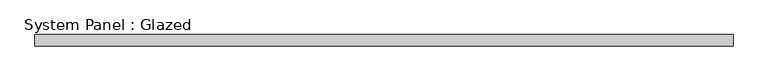
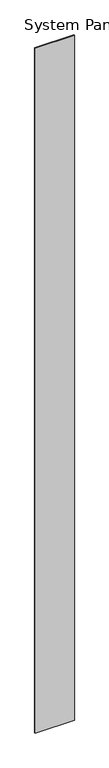
"""IFC4 building model written with IfcOpenShell, lengths in millimetres: plate geometry, System Panel : Glazed."""

from ifc_helpers import new_model, si_unit, origin, origin_with_axes, place, context, project, spatial, polyline, outline, extrude, source, transform, mapped, element, save


def system_panel_glazed_c7023cb4(model_context):
    return source(origin(), model_context, "Body", "SweptSolid", [
        extrude(outline(polyline([(790.575, 19.05), (-790.575, 19.05), (-790.575, 44.45), (790.575, 44.45), (790.575, 19.05)])), origin_with_axes(), (0.0, 0.0, 1.0), 29133.8),
    ])


if __name__ == "__main__":
    model = new_model("IFC4")
    model_context = context("Model", 3, world=origin())
    ifc_project = project(units=[si_unit("LENGTHUNIT", "METRE", prefix="MILLI")], contexts=[model_context])
    site = spatial("IfcSite", under=ifc_project)
    building = spatial("IfcBuilding", under=site)
    placement = place(None, origin())
    system_panel_glazed_shape = system_panel_glazed_c7023cb4(model_context)
    element("IfcPlate", 1, ObjectType="System Panel : Glazed", at=placement, inside=building, context=model_context, shape_type="MappedRepresentation", body=[
        mapped(system_panel_glazed_shape, transform((0.0, 0.0, 0.0), x_axis=(1.0, 0.0, 0.0), y_axis=(0.0, 1.0, 0.0), z_axis=(0.0, 0.0, 1.0))),
    ])
    save(model, "model.ifc")

# Revit data of these elements
# Type "System Panel : Glazed"
#   Construction Type Id = "GSP4R"
#   Analytic Construction = "1/8 in Pilkington single glazing"
#   Visual Light Transmittance = 0.9
#   Solar Heat Gain Coefficient = 0.86
#   Heat Transfer Coefficient (U) = 1.18115 BTU/(h·ft²·°F)
# Element 1 (IfcPlate, "System Panel : Glazed")
#   Materials on its faces: "Glass"
# Materials
#   "Glass": class "Glass", colour RGB 0 128 192, transparency 0.75, Description = "Soda Lime Glass", Cost = 0
